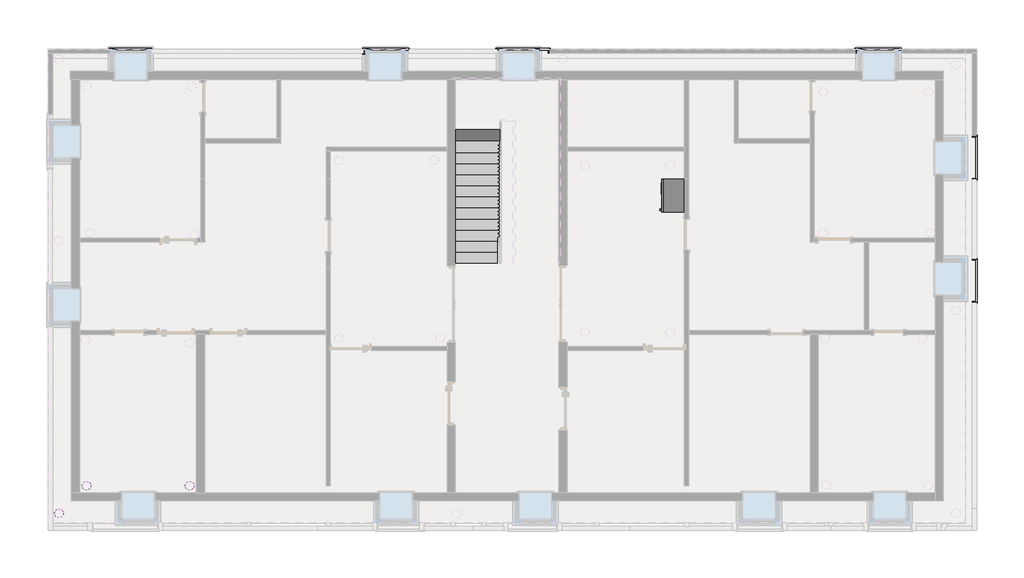
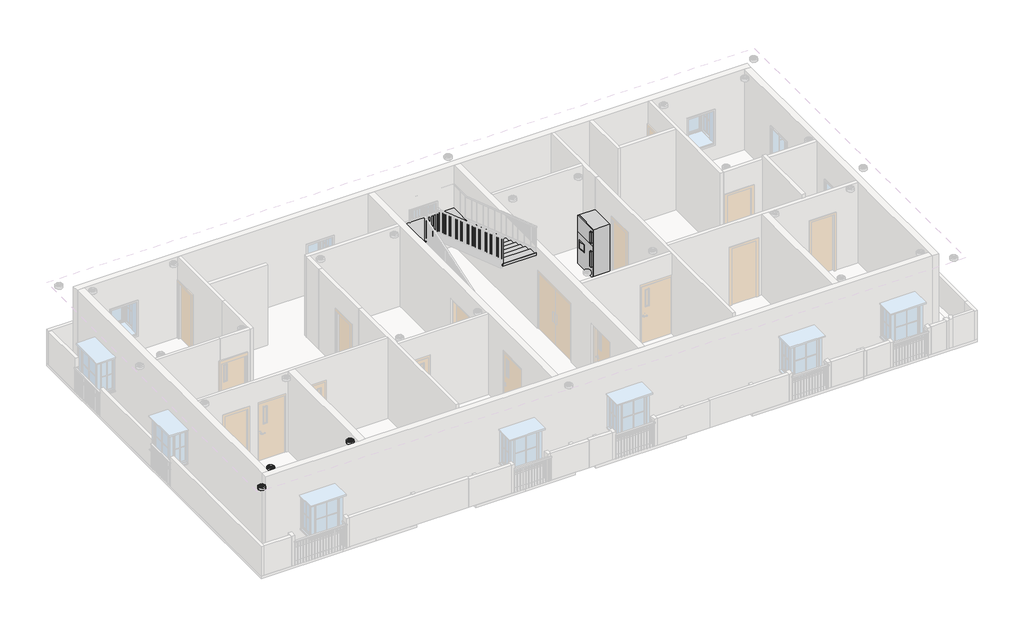
# One storey, part 6 of 7: 6 railings, 3 light fixtures, 1 furniture element, 1 stair flight.
"""IFC4 building model written with IfcOpenShell, lengths in millimetres."""

from ifc_helpers import new_model, si_unit, frame, origin, place, context, project, spatial, polyline, outline, extrude, faceted_brep, transform, mapped, element, save
from components import furniture_65fa61b5, ceiling_light_flat_round_60w_120v_7c4c2a52, stair_flight_b42c0417

model = new_model("IFC4")

# Units and contexts
model_context = context("Model", 3, world=origin())
ifc_project = project(units=[si_unit("LENGTHUNIT", "METRE", prefix="MILLI")], contexts=[model_context])

# Site, building, storey
site = spatial("IfcSite", under=ifc_project)
building = spatial("IfcBuilding", under=site)
storey = spatial("IfcBuildingStorey", under=building, Elevation=3200.4)

# Furniture
placement = place(None, origin())
furniture_shape = furniture_65fa61b5(model_context)
element("IfcFurniture", 1, at=placement, inside=storey, context=model_context, shape_type="MappedRepresentation", body=[
    mapped(furniture_shape, transform((4507.551208, 3815.4567334, 3200.4), x_axis=(0.0, -1.0, 0.0), y_axis=(1.0, 0.0, 0.0), z_axis=(0.0, 0.0, 1.0))),
])

# Light fixtures
ceiling_light_flat_round_60w_120v_shape = ceiling_light_flat_round_60w_120v_7c4c2a52(model_context)
element("IfcLightFixture", 2, ObjectType="Ceiling Light - Flat Round : 60W - 120V", at=placement, inside=storey, context=model_context, shape_type="MappedRepresentation", body=[
    mapped(ceiling_light_flat_round_60w_120v_shape, transform((-12796.1987925, -4356.9932193, 3810.0), x_axis=(1.0, 0.0, 0.0), y_axis=(0.0, 1.0, 0.0), z_axis=(0.0, 0.0, 1.0))),
])
element("IfcLightFixture", 3, ObjectType="Ceiling Light - Flat Round : 60W - 120V", at=placement, inside=storey, context=model_context, shape_type="MappedRepresentation", body=[
    mapped(ceiling_light_flat_round_60w_120v_shape, transform((-12034.1987925, -3594.9932193, 3810.0), x_axis=(1.0, 0.0, 0.0), y_axis=(0.0, 1.0, 0.0), z_axis=(0.0, 0.0, 1.0))),
])
element("IfcLightFixture", 4, ObjectType="Ceiling Light - Flat Round : 60W - 120V", at=placement, inside=storey, context=model_context, shape_type="MappedRepresentation", body=[
    mapped(ceiling_light_flat_round_60w_120v_shape, transform((-9189.3987992, -3594.9932193, 3810.0), x_axis=(1.0, 0.0, 0.0), y_axis=(0.0, 1.0, 0.0), z_axis=(0.0, 0.0, 1.0))),
])

# Railings
element("IfcRailing", 5, ObjectType="Handrail - Rectangular", at=placement, inside=storey, context=model_context, shape_type="SolidModel", body=[
    faceted_brep([(-11412.4067989, 8355.7067329, 4114.8), (-11412.4067989, 8355.7067329, 4064.0), (-11361.6067989, 8355.7067329, 4064.0), (-11361.6067989, 8355.7067329, 4114.8), (-11412.4067989, 8495.4067329, 4114.8), (-11412.4067989, 8495.4067329, 4064.0), (-11361.6067989, 8444.6067329, 4064.0), (-11361.6067989, 8444.6067329, 4114.8), (-10231.3067989, 8495.4067329, 4114.8), (-10231.3067989, 8495.4067329, 4064.0), (-10282.1067989, 8444.6067329, 4064.0), (-10282.1067989, 8444.6067329, 4114.8), (-10231.3067989, 8368.4067329, 4114.8), (-10282.1067989, 8368.4067329, 4114.8), (-10282.1067989, 8368.4067329, 4064.0), (-10231.3067989, 8368.4067329, 4064.0)], [[[0, 1, 2, 3]], [[1, 0, 4, 5]], [[2, 1, 5, 6]], [[3, 2, 6, 7]], [[0, 3, 7, 4]], [[5, 4, 8, 9]], [[6, 5, 9, 10]], [[7, 6, 10, 11]], [[4, 7, 11, 8]], [[12, 13, 14, 15]], [[9, 8, 12, 15]], [[10, 9, 15, 14]], [[11, 10, 14, 13]], [[8, 11, 13, 12]]]),
    extrude(outline(polyline([(-10278.9317989, 8460.4817329), (-10278.9317989, 8479.5317329), (-10259.8817989, 8479.5317329), (-10259.8817989, 8460.4817329), (-10278.9317989, 8460.4817329)])), frame((0.0, 0.0, 3200.4), z_axis=(0.0, 0.0, 1.0), x_axis=(1.0, 0.0, 0.0)), (0.0, 0.0, 1.0), 863.6),
    extrude(outline(polyline([(-10380.5317989, 8460.4817329), (-10380.5317989, 8479.5317329), (-10361.4817989, 8479.5317329), (-10361.4817989, 8460.4817329), (-10380.5317989, 8460.4817329)])), frame((0.0, 0.0, 3200.4), z_axis=(0.0, 0.0, 1.0), x_axis=(1.0, 0.0, 0.0)), (0.0, 0.0, 1.0), 863.6),
    extrude(outline(polyline([(-10482.1317989, 8460.4817329), (-10482.1317989, 8479.5317329), (-10463.0817989, 8479.5317329), (-10463.0817989, 8460.4817329), (-10482.1317989, 8460.4817329)])), frame((0.0, 0.0, 3200.4), z_axis=(0.0, 0.0, 1.0), x_axis=(1.0, 0.0, 0.0)), (0.0, 0.0, 1.0), 863.6),
    extrude(outline(polyline([(-10583.7317989, 8460.4817329), (-10583.7317989, 8479.5317329), (-10564.6817989, 8479.5317329), (-10564.6817989, 8460.4817329), (-10583.7317989, 8460.4817329)])), frame((0.0, 0.0, 3200.4), z_axis=(0.0, 0.0, 1.0), x_axis=(1.0, 0.0, 0.0)), (0.0, 0.0, 1.0), 863.6),
    extrude(outline(polyline([(-10685.3317989, 8460.4817329), (-10685.3317989, 8479.5317329), (-10666.2817989, 8479.5317329), (-10666.2817989, 8460.4817329), (-10685.3317989, 8460.4817329)])), frame((0.0, 0.0, 3200.4), z_axis=(0.0, 0.0, 1.0), x_axis=(1.0, 0.0, 0.0)), (0.0, 0.0, 1.0), 863.6),
    extrude(outline(polyline([(-10786.9317989, 8460.4817329), (-10786.9317989, 8479.5317329), (-10767.8817989, 8479.5317329), (-10767.8817989, 8460.4817329), (-10786.9317989, 8460.4817329)])), frame((0.0, 0.0, 3200.4), z_axis=(0.0, 0.0, 1.0), x_axis=(1.0, 0.0, 0.0)), (0.0, 0.0, 1.0), 863.6),
    extrude(outline(polyline([(-10888.5317989, 8460.4817329), (-10888.5317989, 8479.5317329), (-10869.4817989, 8479.5317329), (-10869.4817989, 8460.4817329), (-10888.5317989, 8460.4817329)])), frame((0.0, 0.0, 3200.4), z_axis=(0.0, 0.0, 1.0), x_axis=(1.0, 0.0, 0.0)), (0.0, 0.0, 1.0), 863.6),
    extrude(outline(polyline([(-10990.1317989, 8460.4817329), (-10990.1317989, 8479.5317329), (-10971.0817989, 8479.5317329), (-10971.0817989, 8460.4817329), (-10990.1317989, 8460.4817329)])), frame((0.0, 0.0, 3200.4), z_axis=(0.0, 0.0, 1.0), x_axis=(1.0, 0.0, 0.0)), (0.0, 0.0, 1.0), 863.6),
    extrude(outline(polyline([(-11091.7317989, 8460.4817329), (-11091.7317989, 8479.5317329), (-11072.6817989, 8479.5317329), (-11072.6817989, 8460.4817329), (-11091.7317989, 8460.4817329)])), frame((0.0, 0.0, 3200.4), z_axis=(0.0, 0.0, 1.0), x_axis=(1.0, 0.0, 0.0)), (0.0, 0.0, 1.0), 863.6),
    extrude(outline(polyline([(-11193.3317989, 8460.4817329), (-11193.3317989, 8479.5317329), (-11174.2817989, 8479.5317329), (-11174.2817989, 8460.4817329), (-11193.3317989, 8460.4817329)])), frame((0.0, 0.0, 3200.4), z_axis=(0.0, 0.0, 1.0), x_axis=(1.0, 0.0, 0.0)), (0.0, 0.0, 1.0), 863.6),
    extrude(outline(polyline([(-11294.9317989, 8460.4817329), (-11294.9317989, 8479.5317329), (-11275.8817989, 8479.5317329), (-11275.8817989, 8460.4817329), (-11294.9317989, 8460.4817329)])), frame((0.0, 0.0, 3200.4), z_axis=(0.0, 0.0, 1.0), x_axis=(1.0, 0.0, 0.0)), (0.0, 0.0, 1.0), 863.6),
    extrude(outline(polyline([(-11377.4817989, 8447.7817329), (-11396.5317989, 8447.7817329), (-11396.5317989, 8466.8317329), (-11377.4817989, 8466.8317329), (-11377.4817989, 8447.7817329)])), frame((0.0, 0.0, 3200.4), z_axis=(0.0, 0.0, 1.0), x_axis=(1.0, 0.0, 0.0)), (0.0, 0.0, 1.0), 863.6),
    extrude(outline(polyline([(-10266.2317989, 8460.4817329), (-10266.2317989, 8479.5317329), (-10247.1817989, 8479.5317329), (-10247.1817989, 8460.4817329), (-10266.2317989, 8460.4817329)])), frame((0.0, 0.0, 3200.4), z_axis=(0.0, 0.0, 1.0), x_axis=(1.0, 0.0, 0.0)), (0.0, 0.0, 1.0), 863.6),
    extrude(outline(polyline([(-11377.4817989, 8460.4817329), (-11396.5317989, 8460.4817329), (-11396.5317989, 8479.5317329), (-11377.4817989, 8479.5317329), (-11377.4817989, 8460.4817329)])), frame((0.0, 0.0, 3200.4), z_axis=(0.0, 0.0, 1.0), x_axis=(1.0, 0.0, 0.0)), (0.0, 0.0, 1.0), 863.6),
    extrude(outline(polyline([(-10266.2317989, 8387.4567329), (-10247.1817989, 8387.4567329), (-10247.1817989, 8368.4067329), (-10266.2317989, 8368.4067329), (-10266.2317989, 8387.4567329)])), frame((0.0, 0.0, 3200.4), z_axis=(0.0, 0.0, 1.0), x_axis=(1.0, 0.0, 0.0)), (0.0, 0.0, 1.0), 863.6),
    extrude(outline(polyline([(-11377.4817989, 8355.7067329), (-11396.5317989, 8355.7067329), (-11396.5317989, 8374.7567329), (-11377.4817989, 8374.7567329), (-11377.4817989, 8355.7067329)])), frame((0.0, 0.0, 3200.4), z_axis=(0.0, 0.0, 1.0), x_axis=(1.0, 0.0, 0.0)), (0.0, 0.0, 1.0), 863.6),
])
element("IfcRailing", 6, ObjectType="Handrail - Rectangular", at=placement, inside=storey, context=model_context, shape_type="SolidModel", body=[
    faceted_brep([(-4407.8487992, 8336.6567329, 4114.8), (-4407.8487992, 8336.6567329, 4064.0), (-4357.0487992, 8336.6567329, 4064.0), (-4357.0487992, 8336.6567329, 4114.8), (-4407.8487992, 8495.4067329, 4114.8), (-4407.8487992, 8495.4067329, 4064.0), (-4357.0487992, 8444.6067329, 4064.0), (-4357.0487992, 8444.6067329, 4114.8), (-3120.4490672, 8495.4067329, 4114.8), (-3120.4490672, 8444.6067329, 4114.8), (-3120.4490672, 8444.6067329, 4064.0), (-3120.4490672, 8495.4067329, 4064.0)], [[[0, 1, 2, 3]], [[1, 0, 4, 5]], [[2, 1, 5, 6]], [[3, 2, 6, 7]], [[0, 3, 7, 4]], [[8, 9, 10, 11]], [[5, 4, 8, 11]], [[6, 5, 11, 10]], [[7, 6, 10, 9]], [[4, 7, 9, 8]]]),
    extrude(outline(polyline([(-3172.7737992, 8460.4817329), (-3172.7737992, 8479.5317329), (-3153.7237992, 8479.5317329), (-3153.7237992, 8460.4817329), (-3172.7737992, 8460.4817329)])), frame((0.0, 0.0, 3200.4), z_axis=(0.0, 0.0, 1.0), x_axis=(1.0, 0.0, 0.0)), (0.0, 0.0, 1.0), 863.6),
    extrude(outline(polyline([(-3274.3737992, 8460.4817329), (-3274.3737992, 8479.5317329), (-3255.3237992, 8479.5317329), (-3255.3237992, 8460.4817329), (-3274.3737992, 8460.4817329)])), frame((0.0, 0.0, 3200.4), z_axis=(0.0, 0.0, 1.0), x_axis=(1.0, 0.0, 0.0)), (0.0, 0.0, 1.0), 863.6),
    extrude(outline(polyline([(-3375.9737992, 8460.4817329), (-3375.9737992, 8479.5317329), (-3356.9237992, 8479.5317329), (-3356.9237992, 8460.4817329), (-3375.9737992, 8460.4817329)])), frame((0.0, 0.0, 3200.4), z_axis=(0.0, 0.0, 1.0), x_axis=(1.0, 0.0, 0.0)), (0.0, 0.0, 1.0), 863.6),
    extrude(outline(polyline([(-3477.5737992, 8460.4817329), (-3477.5737992, 8479.5317329), (-3458.5237992, 8479.5317329), (-3458.5237992, 8460.4817329), (-3477.5737992, 8460.4817329)])), frame((0.0, 0.0, 3200.4), z_axis=(0.0, 0.0, 1.0), x_axis=(1.0, 0.0, 0.0)), (0.0, 0.0, 1.0), 863.6),
    extrude(outline(polyline([(-3579.1737992, 8460.4817329), (-3579.1737992, 8479.5317329), (-3560.1237992, 8479.5317329), (-3560.1237992, 8460.4817329), (-3579.1737992, 8460.4817329)])), frame((0.0, 0.0, 3200.4), z_axis=(0.0, 0.0, 1.0), x_axis=(1.0, 0.0, 0.0)), (0.0, 0.0, 1.0), 863.6),
    extrude(outline(polyline([(-3680.7737992, 8460.4817329), (-3680.7737992, 8479.5317329), (-3661.7237992, 8479.5317329), (-3661.7237992, 8460.4817329), (-3680.7737992, 8460.4817329)])), frame((0.0, 0.0, 3200.4), z_axis=(0.0, 0.0, 1.0), x_axis=(1.0, 0.0, 0.0)), (0.0, 0.0, 1.0), 863.6),
    extrude(outline(polyline([(-3782.3737992, 8460.4817329), (-3782.3737992, 8479.5317329), (-3763.3237992, 8479.5317329), (-3763.3237992, 8460.4817329), (-3782.3737992, 8460.4817329)])), frame((0.0, 0.0, 3200.4), z_axis=(0.0, 0.0, 1.0), x_axis=(1.0, 0.0, 0.0)), (0.0, 0.0, 1.0), 863.6),
    extrude(outline(polyline([(-3883.9737992, 8460.4817329), (-3883.9737992, 8479.5317329), (-3864.9237992, 8479.5317329), (-3864.9237992, 8460.4817329), (-3883.9737992, 8460.4817329)])), frame((0.0, 0.0, 3200.4), z_axis=(0.0, 0.0, 1.0), x_axis=(1.0, 0.0, 0.0)), (0.0, 0.0, 1.0), 863.6),
    extrude(outline(polyline([(-3985.5737992, 8460.4817329), (-3985.5737992, 8479.5317329), (-3966.5237992, 8479.5317329), (-3966.5237992, 8460.4817329), (-3985.5737992, 8460.4817329)])), frame((0.0, 0.0, 3200.4), z_axis=(0.0, 0.0, 1.0), x_axis=(1.0, 0.0, 0.0)), (0.0, 0.0, 1.0), 863.6),
    extrude(outline(polyline([(-4087.1737992, 8460.4817329), (-4087.1737992, 8479.5317329), (-4068.1237992, 8479.5317329), (-4068.1237992, 8460.4817329), (-4087.1737992, 8460.4817329)])), frame((0.0, 0.0, 3200.4), z_axis=(0.0, 0.0, 1.0), x_axis=(1.0, 0.0, 0.0)), (0.0, 0.0, 1.0), 863.6),
    extrude(outline(polyline([(-4188.7737992, 8460.4817329), (-4188.7737992, 8479.5317329), (-4169.7237992, 8479.5317329), (-4169.7237992, 8460.4817329), (-4188.7737992, 8460.4817329)])), frame((0.0, 0.0, 3200.4), z_axis=(0.0, 0.0, 1.0), x_axis=(1.0, 0.0, 0.0)), (0.0, 0.0, 1.0), 863.6),
    extrude(outline(polyline([(-4290.3737992, 8460.4817329), (-4290.3737992, 8479.5317329), (-4271.3237992, 8479.5317329), (-4271.3237992, 8460.4817329), (-4290.3737992, 8460.4817329)])), frame((0.0, 0.0, 3200.4), z_axis=(0.0, 0.0, 1.0), x_axis=(1.0, 0.0, 0.0)), (0.0, 0.0, 1.0), 863.6),
    extrude(outline(polyline([(-4372.9237992, 8428.7317329), (-4391.9737992, 8428.7317329), (-4391.9737992, 8447.7817329), (-4372.9237992, 8447.7817329), (-4372.9237992, 8428.7317329)])), frame((0.0, 0.0, 3200.4), z_axis=(0.0, 0.0, 1.0), x_axis=(1.0, 0.0, 0.0)), (0.0, 0.0, 1.0), 863.6),
    extrude(outline(polyline([(-4372.9237992, 8460.4817329), (-4391.9737992, 8460.4817329), (-4391.9737992, 8479.5317329), (-4372.9237992, 8479.5317329), (-4372.9237992, 8460.4817329)])), frame((0.0, 0.0, 3200.4), z_axis=(0.0, 0.0, 1.0), x_axis=(1.0, 0.0, 0.0)), (0.0, 0.0, 1.0), 863.6),
    extrude(outline(polyline([(-3139.4990672, 8460.4817329), (-3139.4990672, 8479.5317329), (-3120.4490672, 8479.5317329), (-3120.4490672, 8460.4817329), (-3139.4990672, 8460.4817329)])), frame((0.0, 0.0, 3200.4), z_axis=(0.0, 0.0, 1.0), x_axis=(1.0, 0.0, 0.0)), (0.0, 0.0, 1.0), 863.6),
    extrude(outline(polyline([(-4372.9237992, 8336.6567329), (-4391.9737992, 8336.6567329), (-4391.9737992, 8355.7067329), (-4372.9237992, 8355.7067329), (-4372.9237992, 8336.6567329)])), frame((0.0, 0.0, 3200.4), z_axis=(0.0, 0.0, 1.0), x_axis=(1.0, 0.0, 0.0)), (0.0, 0.0, 1.0), 863.6),
])
element("IfcRailing", 7, ObjectType="Handrail - Rectangular", at=placement, inside=storey, context=model_context, shape_type="SolidModel", body=[
    faceted_brep([(-732.8490672, 8355.7067329, 4114.8), (-732.8490672, 8355.7067329, 4064.0), (-682.0490672, 8355.7067329, 4064.0), (-682.0490672, 8355.7067329, 4114.8), (-732.8490672, 8495.4067329, 4114.8), (-732.8490672, 8495.4067329, 4064.0), (-682.0490672, 8444.6067329, 4064.0), (-682.0490672, 8444.6067329, 4114.8), (766.8932011, 8495.4067329, 4114.8), (766.8932011, 8495.4067329, 4064.0), (716.0932011, 8444.6067329, 4064.0), (716.0932011, 8444.6067329, 4114.8), (766.8932011, 8355.7067329, 4114.8), (716.0932011, 8355.7067329, 4114.8), (716.0932011, 8355.7067329, 4064.0), (766.8932011, 8355.7067329, 4064.0)], [[[0, 1, 2, 3]], [[1, 0, 4, 5]], [[2, 1, 5, 6]], [[3, 2, 6, 7]], [[0, 3, 7, 4]], [[5, 4, 8, 9]], [[6, 5, 9, 10]], [[7, 6, 10, 11]], [[4, 7, 11, 8]], [[12, 13, 14, 15]], [[9, 8, 12, 15]], [[10, 9, 15, 14]], [[11, 10, 14, 13]], [[8, 11, 13, 12]]]),
    extrude(outline(polyline([(731.9682011, 8377.9317329), (751.0182011, 8377.9317329), (751.0182011, 8358.8817329), (731.9682011, 8358.8817329), (731.9682011, 8377.9317329)])), frame((0.0, 0.0, 3200.4), z_axis=(0.0, 0.0, 1.0), x_axis=(1.0, 0.0, 0.0)), (0.0, 0.0, 1.0), 863.6),
    extrude(outline(polyline([(705.4259328, 8460.4817329), (705.4259328, 8479.5317329), (724.4759328, 8479.5317329), (724.4759328, 8460.4817329), (705.4259328, 8460.4817329)])), frame((0.0, 0.0, 3200.4), z_axis=(0.0, 0.0, 1.0), x_axis=(1.0, 0.0, 0.0)), (0.0, 0.0, 1.0), 863.6),
    extrude(outline(polyline([(603.8259328, 8460.4817329), (603.8259328, 8479.5317329), (622.8759328, 8479.5317329), (622.8759328, 8460.4817329), (603.8259328, 8460.4817329)])), frame((0.0, 0.0, 3200.4), z_axis=(0.0, 0.0, 1.0), x_axis=(1.0, 0.0, 0.0)), (0.0, 0.0, 1.0), 863.6),
    extrude(outline(polyline([(502.2259328, 8460.4817329), (502.2259328, 8479.5317329), (521.2759328, 8479.5317329), (521.2759328, 8460.4817329), (502.2259328, 8460.4817329)])), frame((0.0, 0.0, 3200.4), z_axis=(0.0, 0.0, 1.0), x_axis=(1.0, 0.0, 0.0)), (0.0, 0.0, 1.0), 863.6),
    extrude(outline(polyline([(400.6259328, 8460.4817329), (400.6259328, 8479.5317329), (419.6759328, 8479.5317329), (419.6759328, 8460.4817329), (400.6259328, 8460.4817329)])), frame((0.0, 0.0, 3200.4), z_axis=(0.0, 0.0, 1.0), x_axis=(1.0, 0.0, 0.0)), (0.0, 0.0, 1.0), 863.6),
    extrude(outline(polyline([(299.0259328, 8460.4817329), (299.0259328, 8479.5317329), (318.0759328, 8479.5317329), (318.0759328, 8460.4817329), (299.0259328, 8460.4817329)])), frame((0.0, 0.0, 3200.4), z_axis=(0.0, 0.0, 1.0), x_axis=(1.0, 0.0, 0.0)), (0.0, 0.0, 1.0), 863.6),
    extrude(outline(polyline([(197.4259328, 8460.4817329), (197.4259328, 8479.5317329), (216.4759328, 8479.5317329), (216.4759328, 8460.4817329), (197.4259328, 8460.4817329)])), frame((0.0, 0.0, 3200.4), z_axis=(0.0, 0.0, 1.0), x_axis=(1.0, 0.0, 0.0)), (0.0, 0.0, 1.0), 863.6),
    extrude(outline(polyline([(95.8259328, 8460.4817329), (95.8259328, 8479.5317329), (114.8759328, 8479.5317329), (114.8759328, 8460.4817329), (95.8259328, 8460.4817329)])), frame((0.0, 0.0, 3200.4), z_axis=(0.0, 0.0, 1.0), x_axis=(1.0, 0.0, 0.0)), (0.0, 0.0, 1.0), 863.6),
    extrude(outline(polyline([(-5.7740672, 8460.4817329), (-5.7740672, 8479.5317329), (13.2759328, 8479.5317329), (13.2759328, 8460.4817329), (-5.7740672, 8460.4817329)])), frame((0.0, 0.0, 3200.4), z_axis=(0.0, 0.0, 1.0), x_axis=(1.0, 0.0, 0.0)), (0.0, 0.0, 1.0), 863.6),
    extrude(outline(polyline([(-107.3740672, 8460.4817329), (-107.3740672, 8479.5317329), (-88.3240672, 8479.5317329), (-88.3240672, 8460.4817329), (-107.3740672, 8460.4817329)])), frame((0.0, 0.0, 3200.4), z_axis=(0.0, 0.0, 1.0), x_axis=(1.0, 0.0, 0.0)), (0.0, 0.0, 1.0), 863.6),
    extrude(outline(polyline([(-208.9740672, 8460.4817329), (-208.9740672, 8479.5317329), (-189.9240672, 8479.5317329), (-189.9240672, 8460.4817329), (-208.9740672, 8460.4817329)])), frame((0.0, 0.0, 3200.4), z_axis=(0.0, 0.0, 1.0), x_axis=(1.0, 0.0, 0.0)), (0.0, 0.0, 1.0), 863.6),
    extrude(outline(polyline([(-310.5740672, 8460.4817329), (-310.5740672, 8479.5317329), (-291.5240672, 8479.5317329), (-291.5240672, 8460.4817329), (-310.5740672, 8460.4817329)])), frame((0.0, 0.0, 3200.4), z_axis=(0.0, 0.0, 1.0), x_axis=(1.0, 0.0, 0.0)), (0.0, 0.0, 1.0), 863.6),
    extrude(outline(polyline([(-412.1740672, 8460.4817329), (-412.1740672, 8479.5317329), (-393.1240672, 8479.5317329), (-393.1240672, 8460.4817329), (-412.1740672, 8460.4817329)])), frame((0.0, 0.0, 3200.4), z_axis=(0.0, 0.0, 1.0), x_axis=(1.0, 0.0, 0.0)), (0.0, 0.0, 1.0), 863.6),
    extrude(outline(polyline([(-513.7740672, 8460.4817329), (-513.7740672, 8479.5317329), (-494.7240672, 8479.5317329), (-494.7240672, 8460.4817329), (-513.7740672, 8460.4817329)])), frame((0.0, 0.0, 3200.4), z_axis=(0.0, 0.0, 1.0), x_axis=(1.0, 0.0, 0.0)), (0.0, 0.0, 1.0), 863.6),
    extrude(outline(polyline([(-615.3740672, 8460.4817329), (-615.3740672, 8479.5317329), (-596.3240672, 8479.5317329), (-596.3240672, 8460.4817329), (-615.3740672, 8460.4817329)])), frame((0.0, 0.0, 3200.4), z_axis=(0.0, 0.0, 1.0), x_axis=(1.0, 0.0, 0.0)), (0.0, 0.0, 1.0), 863.6),
    extrude(outline(polyline([(-697.9240672, 8447.7817329), (-716.9740672, 8447.7817329), (-716.9740672, 8466.8317329), (-697.9240672, 8466.8317329), (-697.9240672, 8447.7817329)])), frame((0.0, 0.0, 3200.4), z_axis=(0.0, 0.0, 1.0), x_axis=(1.0, 0.0, 0.0)), (0.0, 0.0, 1.0), 863.6),
    extrude(outline(polyline([(731.9682011, 8460.4817329), (731.9682011, 8479.5317329), (751.0182011, 8479.5317329), (751.0182011, 8460.4817329), (731.9682011, 8460.4817329)])), frame((0.0, 0.0, 3200.4), z_axis=(0.0, 0.0, 1.0), x_axis=(1.0, 0.0, 0.0)), (0.0, 0.0, 1.0), 863.6),
    extrude(outline(polyline([(-697.9240672, 8460.4817329), (-716.9740672, 8460.4817329), (-716.9740672, 8479.5317329), (-697.9240672, 8479.5317329), (-697.9240672, 8460.4817329)])), frame((0.0, 0.0, 3200.4), z_axis=(0.0, 0.0, 1.0), x_axis=(1.0, 0.0, 0.0)), (0.0, 0.0, 1.0), 863.6),
    extrude(outline(polyline([(731.9682011, 8374.7567329), (751.0182011, 8374.7567329), (751.0182011, 8355.7067329), (731.9682011, 8355.7067329), (731.9682011, 8374.7567329)])), frame((0.0, 0.0, 3200.4), z_axis=(0.0, 0.0, 1.0), x_axis=(1.0, 0.0, 0.0)), (0.0, 0.0, 1.0), 863.6),
    extrude(outline(polyline([(-697.9240672, 8355.7067329), (-716.9740672, 8355.7067329), (-716.9740672, 8374.7567329), (-697.9240672, 8374.7567329), (-697.9240672, 8355.7067329)])), frame((0.0, 0.0, 3200.4), z_axis=(0.0, 0.0, 1.0), x_axis=(1.0, 0.0, 0.0)), (0.0, 0.0, 1.0), 863.6),
])
element("IfcRailing", 8, ObjectType="Handrail - Rectangular", at=placement, inside=storey, context=model_context, shape_type="SolidModel", body=[
    faceted_brep([(9174.2932011, 8355.7067329, 4114.8), (9174.2932011, 8355.7067329, 4064.0), (9225.0932011, 8355.7067329, 4064.0), (9225.0932011, 8355.7067329, 4114.8), (9174.2932011, 8495.4067329, 4114.8), (9174.2932011, 8495.4067329, 4064.0), (9225.0932011, 8444.6067329, 4064.0), (9225.0932011, 8444.6067329, 4114.8), (10462.2009401, 8495.4067329, 4114.8), (10462.2009401, 8444.6067329, 4114.8), (10462.2009401, 8444.6067329, 4064.0), (10462.2009401, 8495.4067329, 4064.0)], [[[0, 1, 2, 3]], [[1, 0, 4, 5]], [[2, 1, 5, 6]], [[3, 2, 6, 7]], [[0, 3, 7, 4]], [[8, 9, 10, 11]], [[5, 4, 8, 11]], [[6, 5, 11, 10]], [[7, 6, 10, 9]], [[4, 7, 9, 8]]]),
    extrude(outline(polyline([(10409.3682011, 8460.4817329), (10409.3682011, 8479.5317329), (10428.4182011, 8479.5317329), (10428.4182011, 8460.4817329), (10409.3682011, 8460.4817329)])), frame((0.0, 0.0, 3200.4), z_axis=(0.0, 0.0, 1.0), x_axis=(1.0, 0.0, 0.0)), (0.0, 0.0, 1.0), 863.6),
    extrude(outline(polyline([(10307.7682011, 8460.4817329), (10307.7682011, 8479.5317329), (10326.8182011, 8479.5317329), (10326.8182011, 8460.4817329), (10307.7682011, 8460.4817329)])), frame((0.0, 0.0, 3200.4), z_axis=(0.0, 0.0, 1.0), x_axis=(1.0, 0.0, 0.0)), (0.0, 0.0, 1.0), 863.6),
    extrude(outline(polyline([(10206.1682011, 8460.4817329), (10206.1682011, 8479.5317329), (10225.2182011, 8479.5317329), (10225.2182011, 8460.4817329), (10206.1682011, 8460.4817329)])), frame((0.0, 0.0, 3200.4), z_axis=(0.0, 0.0, 1.0), x_axis=(1.0, 0.0, 0.0)), (0.0, 0.0, 1.0), 863.6),
    extrude(outline(polyline([(10104.5682011, 8460.4817329), (10104.5682011, 8479.5317329), (10123.6182011, 8479.5317329), (10123.6182011, 8460.4817329), (10104.5682011, 8460.4817329)])), frame((0.0, 0.0, 3200.4), z_axis=(0.0, 0.0, 1.0), x_axis=(1.0, 0.0, 0.0)), (0.0, 0.0, 1.0), 863.6),
    extrude(outline(polyline([(10002.9682011, 8460.4817329), (10002.9682011, 8479.5317329), (10022.0182011, 8479.5317329), (10022.0182011, 8460.4817329), (10002.9682011, 8460.4817329)])), frame((0.0, 0.0, 3200.4), z_axis=(0.0, 0.0, 1.0), x_axis=(1.0, 0.0, 0.0)), (0.0, 0.0, 1.0), 863.6),
    extrude(outline(polyline([(9901.3682011, 8460.4817329), (9901.3682011, 8479.5317329), (9920.4182011, 8479.5317329), (9920.4182011, 8460.4817329), (9901.3682011, 8460.4817329)])), frame((0.0, 0.0, 3200.4), z_axis=(0.0, 0.0, 1.0), x_axis=(1.0, 0.0, 0.0)), (0.0, 0.0, 1.0), 863.6),
    extrude(outline(polyline([(9799.7682011, 8460.4817329), (9799.7682011, 8479.5317329), (9818.8182011, 8479.5317329), (9818.8182011, 8460.4817329), (9799.7682011, 8460.4817329)])), frame((0.0, 0.0, 3200.4), z_axis=(0.0, 0.0, 1.0), x_axis=(1.0, 0.0, 0.0)), (0.0, 0.0, 1.0), 863.6),
    extrude(outline(polyline([(9698.1682011, 8460.4817329), (9698.1682011, 8479.5317329), (9717.2182011, 8479.5317329), (9717.2182011, 8460.4817329), (9698.1682011, 8460.4817329)])), frame((0.0, 0.0, 3200.4), z_axis=(0.0, 0.0, 1.0), x_axis=(1.0, 0.0, 0.0)), (0.0, 0.0, 1.0), 863.6),
    extrude(outline(polyline([(9596.5682011, 8460.4817329), (9596.5682011, 8479.5317329), (9615.6182011, 8479.5317329), (9615.6182011, 8460.4817329), (9596.5682011, 8460.4817329)])), frame((0.0, 0.0, 3200.4), z_axis=(0.0, 0.0, 1.0), x_axis=(1.0, 0.0, 0.0)), (0.0, 0.0, 1.0), 863.6),
    extrude(outline(polyline([(9494.9682011, 8460.4817329), (9494.9682011, 8479.5317329), (9514.0182011, 8479.5317329), (9514.0182011, 8460.4817329), (9494.9682011, 8460.4817329)])), frame((0.0, 0.0, 3200.4), z_axis=(0.0, 0.0, 1.0), x_axis=(1.0, 0.0, 0.0)), (0.0, 0.0, 1.0), 863.6),
    extrude(outline(polyline([(9393.3682011, 8460.4817329), (9393.3682011, 8479.5317329), (9412.4182011, 8479.5317329), (9412.4182011, 8460.4817329), (9393.3682011, 8460.4817329)])), frame((0.0, 0.0, 3200.4), z_axis=(0.0, 0.0, 1.0), x_axis=(1.0, 0.0, 0.0)), (0.0, 0.0, 1.0), 863.6),
    extrude(outline(polyline([(9291.7682011, 8460.4817329), (9291.7682011, 8479.5317329), (9310.8182011, 8479.5317329), (9310.8182011, 8460.4817329), (9291.7682011, 8460.4817329)])), frame((0.0, 0.0, 3200.4), z_axis=(0.0, 0.0, 1.0), x_axis=(1.0, 0.0, 0.0)), (0.0, 0.0, 1.0), 863.6),
    extrude(outline(polyline([(9209.2182011, 8447.7817329), (9190.1682011, 8447.7817329), (9190.1682011, 8466.8317329), (9209.2182011, 8466.8317329), (9209.2182011, 8447.7817329)])), frame((0.0, 0.0, 3200.4), z_axis=(0.0, 0.0, 1.0), x_axis=(1.0, 0.0, 0.0)), (0.0, 0.0, 1.0), 863.6),
    extrude(outline(polyline([(9209.2182011, 8460.4817329), (9190.1682011, 8460.4817329), (9190.1682011, 8479.5317329), (9209.2182011, 8479.5317329), (9209.2182011, 8460.4817329)])), frame((0.0, 0.0, 3200.4), z_axis=(0.0, 0.0, 1.0), x_axis=(1.0, 0.0, 0.0)), (0.0, 0.0, 1.0), 863.6),
    extrude(outline(polyline([(10443.1509401, 8460.4817329), (10443.1509401, 8479.5317329), (10462.2009401, 8479.5317329), (10462.2009401, 8460.4817329), (10443.1509401, 8460.4817329)])), frame((0.0, 0.0, 3200.4), z_axis=(0.0, 0.0, 1.0), x_axis=(1.0, 0.0, 0.0)), (0.0, 0.0, 1.0), 863.6),
    extrude(outline(polyline([(9209.2182011, 8355.7067329), (9190.1682011, 8355.7067329), (9190.1682011, 8374.7567329), (9209.2182011, 8374.7567329), (9209.2182011, 8355.7067329)])), frame((0.0, 0.0, 3200.4), z_axis=(0.0, 0.0, 1.0), x_axis=(1.0, 0.0, 0.0)), (0.0, 0.0, 1.0), 863.6),
])
element("IfcRailing", 9, ObjectType="Handrail - Rectangular", at=placement, inside=storey, context=model_context, shape_type="SolidModel", body=[
    faceted_brep([(12426.0012043, 2691.5067329, 4114.8), (12426.0012043, 2691.5067329, 4064.0), (12426.0012043, 2640.7067329, 4064.0), (12426.0012043, 2640.7067329, 4114.8), (12565.7012043, 2691.5067329, 4114.8), (12565.7012043, 2691.5067329, 4064.0), (12514.9012043, 2640.7067329, 4064.0), (12514.9012043, 2640.7067329, 4114.8), (12565.7012043, 1453.2567334, 4114.8), (12565.7012043, 1453.2567334, 4064.0), (12514.9012043, 1504.0567334, 4064.0), (12514.9012043, 1504.0567334, 4114.8), (12426.0012043, 1453.2567334, 4114.8), (12426.0012043, 1504.0567334, 4114.8), (12426.0012043, 1504.0567334, 4064.0), (12426.0012043, 1453.2567334, 4064.0)], [[[0, 1, 2, 3]], [[1, 0, 4, 5]], [[2, 1, 5, 6]], [[3, 2, 6, 7]], [[0, 3, 7, 4]], [[5, 4, 8, 9]], [[6, 5, 9, 10]], [[7, 6, 10, 11]], [[4, 7, 11, 8]], [[12, 13, 14, 15]], [[9, 8, 12, 15]], [[10, 9, 15, 14]], [[11, 10, 14, 13]], [[8, 11, 13, 12]]]),
    extrude(outline(polyline([(12448.2262043, 1488.1817334), (12448.2262043, 1469.1317334), (12429.1762043, 1469.1317334), (12429.1762043, 1488.1817334), (12448.2262043, 1488.1817334)])), frame((0.0, 0.0, 3200.4), z_axis=(0.0, 0.0, 1.0), x_axis=(1.0, 0.0, 0.0)), (0.0, 0.0, 1.0), 863.6),
    extrude(outline(polyline([(12530.7762043, 1558.0317329), (12549.8262043, 1558.0317329), (12549.8262043, 1538.9817329), (12530.7762043, 1538.9817329), (12530.7762043, 1558.0317329)])), frame((0.0, 0.0, 3200.4), z_axis=(0.0, 0.0, 1.0), x_axis=(1.0, 0.0, 0.0)), (0.0, 0.0, 1.0), 863.6),
    extrude(outline(polyline([(12530.7762043, 1659.6317329), (12549.8262043, 1659.6317329), (12549.8262043, 1640.5817329), (12530.7762043, 1640.5817329), (12530.7762043, 1659.6317329)])), frame((0.0, 0.0, 3200.4), z_axis=(0.0, 0.0, 1.0), x_axis=(1.0, 0.0, 0.0)), (0.0, 0.0, 1.0), 863.6),
    extrude(outline(polyline([(12530.7762043, 1761.2317329), (12549.8262043, 1761.2317329), (12549.8262043, 1742.1817329), (12530.7762043, 1742.1817329), (12530.7762043, 1761.2317329)])), frame((0.0, 0.0, 3200.4), z_axis=(0.0, 0.0, 1.0), x_axis=(1.0, 0.0, 0.0)), (0.0, 0.0, 1.0), 863.6),
    extrude(outline(polyline([(12530.7762043, 1862.8317329), (12549.8262043, 1862.8317329), (12549.8262043, 1843.7817329), (12530.7762043, 1843.7817329), (12530.7762043, 1862.8317329)])), frame((0.0, 0.0, 3200.4), z_axis=(0.0, 0.0, 1.0), x_axis=(1.0, 0.0, 0.0)), (0.0, 0.0, 1.0), 863.6),
    extrude(outline(polyline([(12530.7762043, 1964.4317329), (12549.8262043, 1964.4317329), (12549.8262043, 1945.3817329), (12530.7762043, 1945.3817329), (12530.7762043, 1964.4317329)])), frame((0.0, 0.0, 3200.4), z_axis=(0.0, 0.0, 1.0), x_axis=(1.0, 0.0, 0.0)), (0.0, 0.0, 1.0), 863.6),
    extrude(outline(polyline([(12530.7762043, 2066.0317329), (12549.8262043, 2066.0317329), (12549.8262043, 2046.9817329), (12530.7762043, 2046.9817329), (12530.7762043, 2066.0317329)])), frame((0.0, 0.0, 3200.4), z_axis=(0.0, 0.0, 1.0), x_axis=(1.0, 0.0, 0.0)), (0.0, 0.0, 1.0), 863.6),
    extrude(outline(polyline([(12530.7762043, 2167.6317329), (12549.8262043, 2167.6317329), (12549.8262043, 2148.5817329), (12530.7762043, 2148.5817329), (12530.7762043, 2167.6317329)])), frame((0.0, 0.0, 3200.4), z_axis=(0.0, 0.0, 1.0), x_axis=(1.0, 0.0, 0.0)), (0.0, 0.0, 1.0), 863.6),
    extrude(outline(polyline([(12530.7762043, 2269.2317329), (12549.8262043, 2269.2317329), (12549.8262043, 2250.1817329), (12530.7762043, 2250.1817329), (12530.7762043, 2269.2317329)])), frame((0.0, 0.0, 3200.4), z_axis=(0.0, 0.0, 1.0), x_axis=(1.0, 0.0, 0.0)), (0.0, 0.0, 1.0), 863.6),
    extrude(outline(polyline([(12530.7762043, 2370.8317329), (12549.8262043, 2370.8317329), (12549.8262043, 2351.7817329), (12530.7762043, 2351.7817329), (12530.7762043, 2370.8317329)])), frame((0.0, 0.0, 3200.4), z_axis=(0.0, 0.0, 1.0), x_axis=(1.0, 0.0, 0.0)), (0.0, 0.0, 1.0), 863.6),
    extrude(outline(polyline([(12530.7762043, 2472.4317329), (12549.8262043, 2472.4317329), (12549.8262043, 2453.3817329), (12530.7762043, 2453.3817329), (12530.7762043, 2472.4317329)])), frame((0.0, 0.0, 3200.4), z_axis=(0.0, 0.0, 1.0), x_axis=(1.0, 0.0, 0.0)), (0.0, 0.0, 1.0), 863.6),
    extrude(outline(polyline([(12530.7762043, 2574.0317329), (12549.8262043, 2574.0317329), (12549.8262043, 2554.9817329), (12530.7762043, 2554.9817329), (12530.7762043, 2574.0317329)])), frame((0.0, 0.0, 3200.4), z_axis=(0.0, 0.0, 1.0), x_axis=(1.0, 0.0, 0.0)), (0.0, 0.0, 1.0), 863.6),
    extrude(outline(polyline([(12518.0762043, 2656.5817329), (12518.0762043, 2675.6317329), (12537.1262043, 2675.6317329), (12537.1262043, 2656.5817329), (12518.0762043, 2656.5817329)])), frame((0.0, 0.0, 3200.4), z_axis=(0.0, 0.0, 1.0), x_axis=(1.0, 0.0, 0.0)), (0.0, 0.0, 1.0), 863.6),
    extrude(outline(polyline([(12530.7762043, 1488.1817334), (12549.8262043, 1488.1817334), (12549.8262043, 1469.1317334), (12530.7762043, 1469.1317334), (12530.7762043, 1488.1817334)])), frame((0.0, 0.0, 3200.4), z_axis=(0.0, 0.0, 1.0), x_axis=(1.0, 0.0, 0.0)), (0.0, 0.0, 1.0), 863.6),
    extrude(outline(polyline([(12530.7762043, 2656.5817329), (12530.7762043, 2675.6317329), (12549.8262043, 2675.6317329), (12549.8262043, 2656.5817329), (12530.7762043, 2656.5817329)])), frame((0.0, 0.0, 3200.4), z_axis=(0.0, 0.0, 1.0), x_axis=(1.0, 0.0, 0.0)), (0.0, 0.0, 1.0), 863.6),
    extrude(outline(polyline([(12445.0512043, 1488.1817334), (12445.0512043, 1469.1317334), (12426.0012043, 1469.1317334), (12426.0012043, 1488.1817334), (12445.0512043, 1488.1817334)])), frame((0.0, 0.0, 3200.4), z_axis=(0.0, 0.0, 1.0), x_axis=(1.0, 0.0, 0.0)), (0.0, 0.0, 1.0), 863.6),
    extrude(outline(polyline([(12426.0012043, 2656.5817329), (12426.0012043, 2675.6317329), (12445.0512043, 2675.6317329), (12445.0512043, 2656.5817329), (12426.0012043, 2656.5817329)])), frame((0.0, 0.0, 3200.4), z_axis=(0.0, 0.0, 1.0), x_axis=(1.0, 0.0, 0.0)), (0.0, 0.0, 1.0), 863.6),
])
element("IfcRailing", 10, ObjectType="Handrail - Rectangular", at=placement, inside=storey, context=model_context, shape_type="SolidModel", body=[
    faceted_brep([(12426.0012043, 6095.1067329, 4114.8), (12426.0012043, 6095.1067329, 4064.0), (12426.0012043, 6044.3067329, 4064.0), (12426.0012043, 6044.3067329, 4114.8), (12565.7012043, 6095.1067329, 4114.8), (12565.7012043, 6095.1067329, 4064.0), (12514.9012043, 6044.3067329, 4064.0), (12514.9012043, 6044.3067329, 4114.8), (12565.7012043, 4850.5067329, 4114.8), (12565.7012043, 4850.5067329, 4064.0), (12514.9012043, 4901.3067329, 4064.0), (12514.9012043, 4901.3067329, 4114.8), (12426.0012043, 4850.5067329, 4114.8), (12426.0012043, 4901.3067329, 4114.8), (12426.0012043, 4901.3067329, 4064.0), (12426.0012043, 4850.5067329, 4064.0)], [[[0, 1, 2, 3]], [[1, 0, 4, 5]], [[2, 1, 5, 6]], [[3, 2, 6, 7]], [[0, 3, 7, 4]], [[5, 4, 8, 9]], [[6, 5, 9, 10]], [[7, 6, 10, 11]], [[4, 7, 11, 8]], [[12, 13, 14, 15]], [[9, 8, 12, 15]], [[10, 9, 15, 14]], [[11, 10, 14, 13]], [[8, 11, 13, 12]]]),
    extrude(outline(polyline([(12448.2262043, 4885.4317329), (12448.2262043, 4866.3817329), (12429.1762043, 4866.3817329), (12429.1762043, 4885.4317329), (12448.2262043, 4885.4317329)])), frame((0.0, 0.0, 3200.4), z_axis=(0.0, 0.0, 1.0), x_axis=(1.0, 0.0, 0.0)), (0.0, 0.0, 1.0), 863.6),
    extrude(outline(polyline([(12530.7762043, 4961.6317329), (12549.8262043, 4961.6317329), (12549.8262043, 4942.5817329), (12530.7762043, 4942.5817329), (12530.7762043, 4961.6317329)])), frame((0.0, 0.0, 3200.4), z_axis=(0.0, 0.0, 1.0), x_axis=(1.0, 0.0, 0.0)), (0.0, 0.0, 1.0), 863.6),
    extrude(outline(polyline([(12530.7762043, 5063.2317329), (12549.8262043, 5063.2317329), (12549.8262043, 5044.1817329), (12530.7762043, 5044.1817329), (12530.7762043, 5063.2317329)])), frame((0.0, 0.0, 3200.4), z_axis=(0.0, 0.0, 1.0), x_axis=(1.0, 0.0, 0.0)), (0.0, 0.0, 1.0), 863.6),
    extrude(outline(polyline([(12530.7762043, 5164.8317329), (12549.8262043, 5164.8317329), (12549.8262043, 5145.7817329), (12530.7762043, 5145.7817329), (12530.7762043, 5164.8317329)])), frame((0.0, 0.0, 3200.4), z_axis=(0.0, 0.0, 1.0), x_axis=(1.0, 0.0, 0.0)), (0.0, 0.0, 1.0), 863.6),
    extrude(outline(polyline([(12530.7762043, 5266.4317329), (12549.8262043, 5266.4317329), (12549.8262043, 5247.3817329), (12530.7762043, 5247.3817329), (12530.7762043, 5266.4317329)])), frame((0.0, 0.0, 3200.4), z_axis=(0.0, 0.0, 1.0), x_axis=(1.0, 0.0, 0.0)), (0.0, 0.0, 1.0), 863.6),
    extrude(outline(polyline([(12530.7762043, 5368.0317329), (12549.8262043, 5368.0317329), (12549.8262043, 5348.9817329), (12530.7762043, 5348.9817329), (12530.7762043, 5368.0317329)])), frame((0.0, 0.0, 3200.4), z_axis=(0.0, 0.0, 1.0), x_axis=(1.0, 0.0, 0.0)), (0.0, 0.0, 1.0), 863.6),
    extrude(outline(polyline([(12530.7762043, 5469.6317329), (12549.8262043, 5469.6317329), (12549.8262043, 5450.5817329), (12530.7762043, 5450.5817329), (12530.7762043, 5469.6317329)])), frame((0.0, 0.0, 3200.4), z_axis=(0.0, 0.0, 1.0), x_axis=(1.0, 0.0, 0.0)), (0.0, 0.0, 1.0), 863.6),
    extrude(outline(polyline([(12530.7762043, 5571.2317329), (12549.8262043, 5571.2317329), (12549.8262043, 5552.1817329), (12530.7762043, 5552.1817329), (12530.7762043, 5571.2317329)])), frame((0.0, 0.0, 3200.4), z_axis=(0.0, 0.0, 1.0), x_axis=(1.0, 0.0, 0.0)), (0.0, 0.0, 1.0), 863.6),
    extrude(outline(polyline([(12530.7762043, 5672.8317329), (12549.8262043, 5672.8317329), (12549.8262043, 5653.7817329), (12530.7762043, 5653.7817329), (12530.7762043, 5672.8317329)])), frame((0.0, 0.0, 3200.4), z_axis=(0.0, 0.0, 1.0), x_axis=(1.0, 0.0, 0.0)), (0.0, 0.0, 1.0), 863.6),
    extrude(outline(polyline([(12530.7762043, 5774.4317329), (12549.8262043, 5774.4317329), (12549.8262043, 5755.3817329), (12530.7762043, 5755.3817329), (12530.7762043, 5774.4317329)])), frame((0.0, 0.0, 3200.4), z_axis=(0.0, 0.0, 1.0), x_axis=(1.0, 0.0, 0.0)), (0.0, 0.0, 1.0), 863.6),
    extrude(outline(polyline([(12530.7762043, 5876.0317329), (12549.8262043, 5876.0317329), (12549.8262043, 5856.9817329), (12530.7762043, 5856.9817329), (12530.7762043, 5876.0317329)])), frame((0.0, 0.0, 3200.4), z_axis=(0.0, 0.0, 1.0), x_axis=(1.0, 0.0, 0.0)), (0.0, 0.0, 1.0), 863.6),
    extrude(outline(polyline([(12530.7762043, 5977.6317329), (12549.8262043, 5977.6317329), (12549.8262043, 5958.5817329), (12530.7762043, 5958.5817329), (12530.7762043, 5977.6317329)])), frame((0.0, 0.0, 3200.4), z_axis=(0.0, 0.0, 1.0), x_axis=(1.0, 0.0, 0.0)), (0.0, 0.0, 1.0), 863.6),
    extrude(outline(polyline([(12518.0762043, 6060.1817329), (12518.0762043, 6079.2317329), (12537.1262043, 6079.2317329), (12537.1262043, 6060.1817329), (12518.0762043, 6060.1817329)])), frame((0.0, 0.0, 3200.4), z_axis=(0.0, 0.0, 1.0), x_axis=(1.0, 0.0, 0.0)), (0.0, 0.0, 1.0), 863.6),
    extrude(outline(polyline([(12530.7762043, 4885.4317329), (12549.8262043, 4885.4317329), (12549.8262043, 4866.3817329), (12530.7762043, 4866.3817329), (12530.7762043, 4885.4317329)])), frame((0.0, 0.0, 3200.4), z_axis=(0.0, 0.0, 1.0), x_axis=(1.0, 0.0, 0.0)), (0.0, 0.0, 1.0), 863.6),
    extrude(outline(polyline([(12530.7762043, 6060.1817329), (12530.7762043, 6079.2317329), (12549.8262043, 6079.2317329), (12549.8262043, 6060.1817329), (12530.7762043, 6060.1817329)])), frame((0.0, 0.0, 3200.4), z_axis=(0.0, 0.0, 1.0), x_axis=(1.0, 0.0, 0.0)), (0.0, 0.0, 1.0), 863.6),
    extrude(outline(polyline([(12445.0512043, 4885.4317329), (12445.0512043, 4866.3817329), (12426.0012043, 4866.3817329), (12426.0012043, 4885.4317329), (12445.0512043, 4885.4317329)])), frame((0.0, 0.0, 3200.4), z_axis=(0.0, 0.0, 1.0), x_axis=(1.0, 0.0, 0.0)), (0.0, 0.0, 1.0), 863.6),
    extrude(outline(polyline([(12426.0012043, 6060.1817329), (12426.0012043, 6079.2317329), (12445.0512043, 6079.2317329), (12445.0512043, 6060.1817329), (12426.0012043, 6060.1817329)])), frame((0.0, 0.0, 3200.4), z_axis=(0.0, 0.0, 1.0), x_axis=(1.0, 0.0, 0.0)), (0.0, 0.0, 1.0), 863.6),
])

# Stair flight
stair_flight_shape = stair_flight_b42c0417(model_context)
element("IfcStairFlight", 11, ObjectType="2\" Tread 1\" Nosing 1/4\" Riser", at=placement, inside=storey, context=model_context, shape_type="MappedRepresentation", body=[
    mapped(stair_flight_shape, transform((0.0, 0.0, 0.0), x_axis=(1.0, 0.0, 0.0), y_axis=(0.0, 1.0, 0.0), z_axis=(0.0, 0.0, 1.0))),
])

save(model, "model.ifc")

# Revit data of these elements
# Type
#   Default Elevation = 0
# Type "Ceiling Light - Flat Round : 60W - 120V"
#   Lamp = "A-19"
#   Assembly Code = "D5020220"
#   Wattage = 60 W
#   built-in parameter 1150110 = 1 (stored number, unit not read)
#   built-in parameter 1114217 = 1 (stored number, unit not read)
#   built-in parameter 1150109 = 1 (stored number, unit not read)
#   built-in parameter 1150113 = 1 (stored number, unit not read)
#   built-in parameter 1150115 = 1 (stored number, unit not read)
#   built-in parameter 1150105 = 272.155 (stored number, unit not read)
#   Light Source Symbol Size = 2' - 0"
#   built-in parameter 1150112 = 1 (stored number, unit not read)
#   built-in parameter 1150114 = 1 (stored number, unit not read)
#   built-in parameter 1150107 = 2800 (stored number, unit not read)
#   built-in parameter 1150106 = 2.72155 (stored number, unit not read)
#   Emit from Circle Diameter = 0' - 10"
#   built-in parameter 1150104 = 1.32387 (stored number, unit not read)
#   Ballast Voltage = 120 V
#   built-in parameter 1114218 = 1 (stored number, unit not read)
#   built-in parameter 1150133 = 10 (stored number, unit not read)
#   Lumens = 855 lm
#   Apparent Load = 60 VA
#   built-in parameter 1150134 = 4
#   built-in parameter 1150137 = 1
#   Color Filter = 16777215
#   built-in parameter 1140040 [instance default] = 1
#   Ballast Number of Poles = 1
#   Light Box Material = Steel, Paint Finish, Dark Gray, Matte
#   Diffuser Material = Glass, White, High Luminance
#   Wattage Comments = ""
#   Emit Shape Visible in Rendering = no
#   Dimming Lamp Color Temperature Shift = (empty or 0)
#   Default Elevation = 0
# Type "Handrail - Rectangular"
#   Assembly Code = "C2010400"
#   built-in parameter 1008612 = 0.0416667 (stored number, unit not read)
#   built-in parameter 1008611 = 0.0416667 (stored number, unit not read)
#   built-in parameter 1008609 = 0.333333 (stored number, unit not read)
#   built-in parameter 1008604 = 0.166667 (stored number, unit not read)
#   built-in parameter 1008603 = 0.166667 (stored number, unit not read)
#   Railing Height = 3' - 0"
#   built-in parameter 1008630 = 2
#   built-in parameter 1008610 = 2
#   built-in parameter 1008618 = Baluster - Square : 3/4"
# Element 1 (IfcFurniture)
#   Phase Created = New Construction
#   Materials on its faces: "Default", "Default 3", "Default 2"
# Element 2 (IfcLightFixture, "Ceiling Light - Flat Round : 60W - 120V")
#   Mark = "30"
#   built-in parameter 1140040 = 1
#   Phase Created = New Construction
#   Materials on its faces: "Glass, White, High Luminance", "Steel, Paint Finish, Dark Gray, Matte"
# Element 3 (IfcLightFixture, "Ceiling Light - Flat Round : 60W - 120V")
#   Mark = "38"
#   built-in parameter 1140040 = 1
#   Phase Created = New Construction
#   Materials on its faces: "Glass, White, High Luminance", "Steel, Paint Finish, Dark Gray, Matte"
# Element 4 (IfcLightFixture, "Ceiling Light - Flat Round : 60W - 120V")
#   Mark = "39"
#   built-in parameter 1140040 = 1
#   Phase Created = New Construction
#   Materials on its faces: "Glass, White, High Luminance", "Steel, Paint Finish, Dark Gray, Matte"
# Elements 5, 6, 7, 8, 9, 10 (IfcRailing, "Handrail - Rectangular")
#   Phase Created = New Construction
# Element 11 (IfcStairFlight, "2\" Tread 1\" Nosing 1/4\" Riser")
#   Phase Created = New Construction
# Materials
#   "Steel, Paint Finish, Dark Gray, Matte": class "Metal", colour RGB 98 98 98, transparency 0, Description = "Steel, paint finish, dark gray, matte", Cost = 0
#   "Glass, White, High Luminance": class "Glass", colour RGB 249 250 249, transparency 0.8, Description = "physical material", Cost = 0
#   "Default": colour RGB 127 127 127, transparency 0, Cost = 0
#   "Default 3": class "Glass", colour RGB 127 127 127, transparency 0
#   "Default 2": class "Plastic", colour RGB 127 127 127, transparency 0
